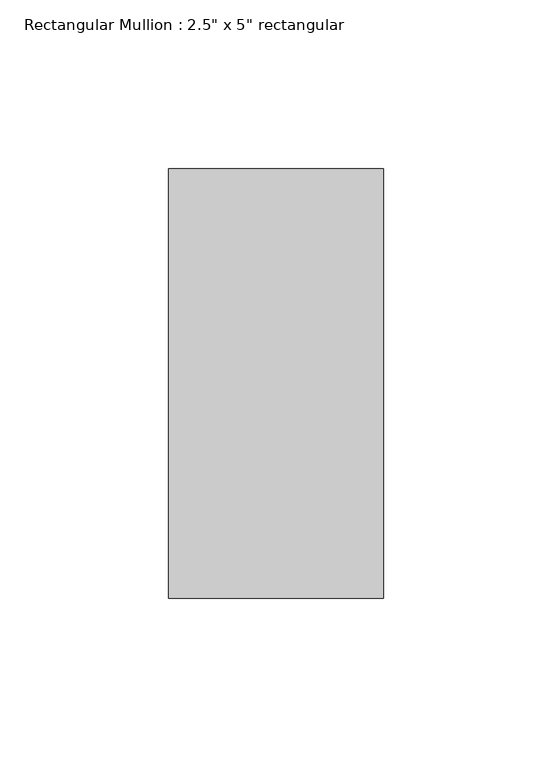
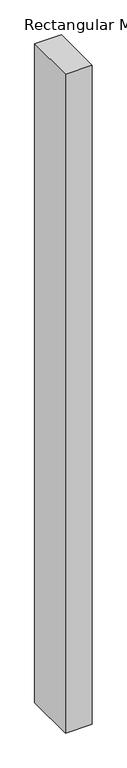
"""IFC4 building model written with IfcOpenShell, lengths in millimetres: member geometry."""

from ifc_helpers import new_model, si_unit, frame, origin, place, context, project, spatial, polyline, outline, extrude, source, transform, mapped, element, save


def member_ac37c43a(model_context):
    return source(origin(), model_context, "Body", "SweptSolid", [
        extrude(outline(polyline([(0.0, 63.5), (0.0, -63.5), (-63.5, -63.5), (-63.5, 63.5), (0.0, 63.5)])), frame((0.0, 0.0, -1659.4287133), z_axis=(0.0, 0.0, 1.0), x_axis=(1.0, 0.0, 0.0)), (0.0, 0.0, 1.0), 1659.4287133),
    ])


if __name__ == "__main__":
    model = new_model("IFC4")
    model_context = context("Model", 3, world=origin())
    ifc_project = project(units=[si_unit("LENGTHUNIT", "METRE", prefix="MILLI")], contexts=[model_context])
    site = spatial("IfcSite", under=ifc_project)
    building = spatial("IfcBuilding", under=site)
    placement = place(None, origin())
    member_shape = member_ac37c43a(model_context)
    element("IfcMember", 1, ObjectType="Rectangular Mullion : 2.5\" x 5\" rectangular", at=placement, inside=building, context=model_context, shape_type="MappedRepresentation", body=[
        mapped(member_shape, transform((0.0, 0.0, 0.0), x_axis=(1.0, 0.0, 0.0), y_axis=(0.0, 1.0, 0.0), z_axis=(0.0, 0.0, 1.0))),
    ])
    save(model, "model.ifc")

# Revit data of these elements
# Type "Rectangular Mullion : 2.5\" x 5\" rectangular"
#   built-in parameter 1007304 = 0.416667 (stored number, unit not read)
#   built-in parameter 1007301 = 0.104167 (stored number, unit not read)
#   built-in parameter 1007300 = 0.104167 (stored number, unit not read)
# Element 1 (IfcMember, "Rectangular Mullion : 2.5\" x 5\" rectangular")
#   Materials on its faces: "Aluminum"
# Materials
#   "Aluminum": class "Metal", colour RGB 247 247 247, transparency 0, Description = "Aluminum 6061", Cost = 0
